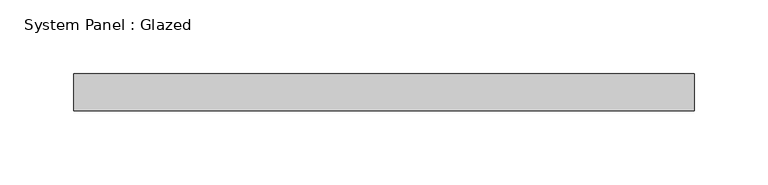
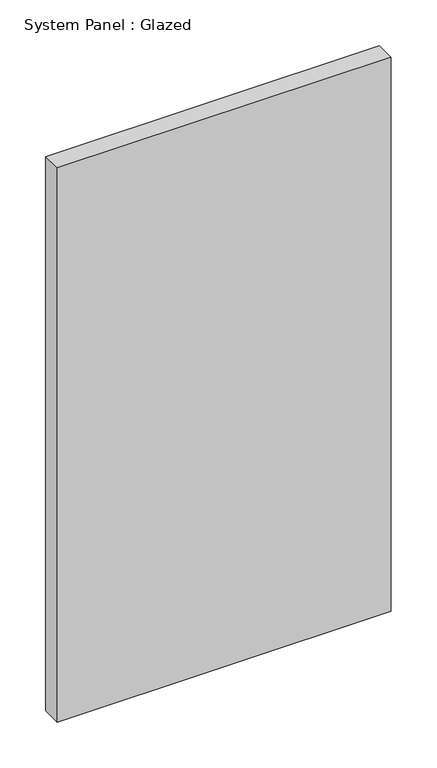
"""IFC4 building model written with IfcOpenShell, lengths in millimetres: plate geometry, System Panel : Glazed."""

from ifc_helpers import new_model, si_unit, origin, origin_with_axes, place, context, project, spatial, polyline, outline, extrude, source, transform, mapped, element, save


def system_panel_glazed_06045eac(model_context):
    return source(origin(), model_context, "Body", "SweptSolid", [
        extrude(outline(polyline([(209.9398924, 24.5), (-209.9398924, 24.5), (-209.9398924, 49.5), (209.9398924, 49.5), (209.9398924, 24.5)])), origin_with_axes(), (0.0, 0.0, 1.0), 736.6),
    ])


if __name__ == "__main__":
    model = new_model("IFC4")
    model_context = context("Model", 3, world=origin())
    ifc_project = project(units=[si_unit("LENGTHUNIT", "METRE", prefix="MILLI")], contexts=[model_context])
    site = spatial("IfcSite", under=ifc_project)
    building = spatial("IfcBuilding", under=site)
    placement = place(None, origin())
    system_panel_glazed_shape = system_panel_glazed_06045eac(model_context)
    element("IfcPlate", 1, ObjectType="System Panel : Glazed", at=placement, inside=building, context=model_context, shape_type="MappedRepresentation", body=[
        mapped(system_panel_glazed_shape, transform((0.0, 0.0, 0.0), x_axis=(1.0, 0.0, 0.0), y_axis=(0.0, 1.0, 0.0), z_axis=(0.0, 0.0, 1.0))),
    ])
    save(model, "model.ifc")

# Revit data of these elements
# Type "System Panel : Glazed"
#   Keynote = "H11"
#   Construction Type Id = "GSP4R"
#   Analytic Construction = "1/8 in Pilkington single glazing"
#   Visual Light Transmittance = 0.9
#   Solar Heat Gain Coefficient = 0.86
#   Heat Transfer Coefficient (U) = 6.7069 W/(m²·K)
#   Define Thermal Properties by = 1
# Element 1 (IfcPlate, "System Panel : Glazed")
#   Materials on its faces: "Glass"
# Materials
#   "Glass": class "Glass", colour RGB 0 128 192, transparency 0.9, Description = "Soda Lime Glass", Cost = 0
